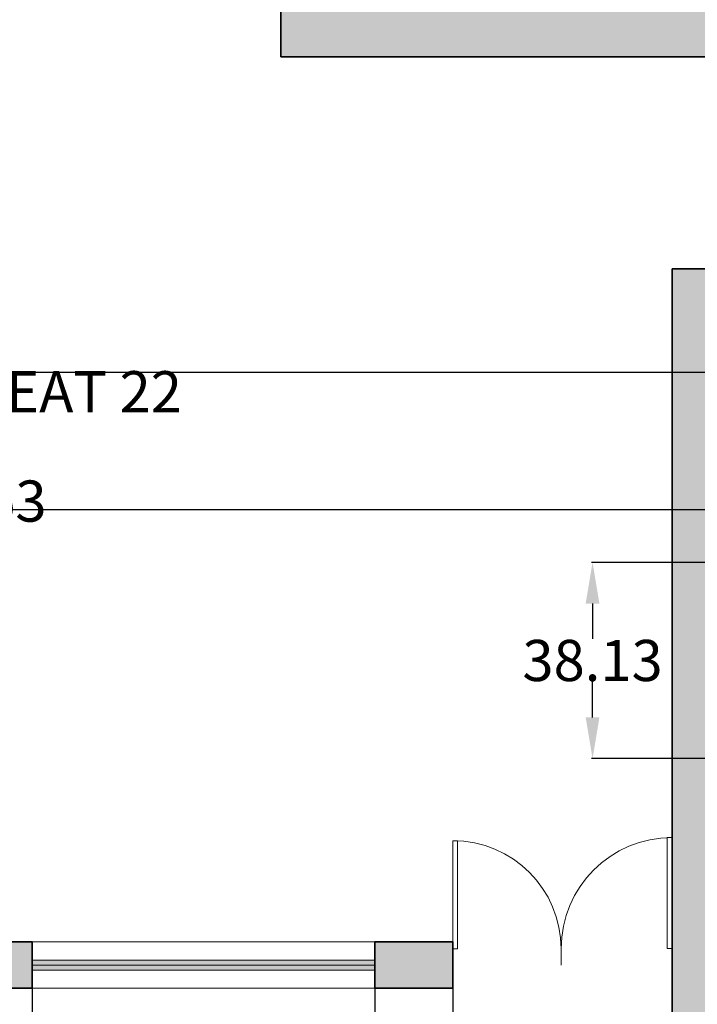
# Model space of a CAD drawing. Units: inches. Extents: x -52 to 678, y 23 to 685.
# Tile 5 of 11: x 299 to 431, y 143 to 334. Entities that reach past the tile are written whole.
import ezdxf

# ---------------------------------------------------------------- set-up
doc = ezdxf.new("R2010")
doc.units = ezdxf.units.IN
doc.header["$MEASUREMENT"] = 0
for name, color, linetype, lineweight in [('A-ANNO-DIMS', 2, 'Continuous', 18), ('A-DOOR', 3, 'Continuous', 18), ('A-GLAZ', 4, 'Continuous', 18), ('A-WALL', 7, 'Continuous', 35)]:
    doc.layers.add(name, color=color, linetype=linetype, lineweight=lineweight)
doc.layers.add('A-GLAZ-PATT', color=18, linetype='Continuous', lineweight=13, true_color=0x000000)
doc.layers.add('A-WALL-PATT', color=18, linetype='Continuous', lineweight=13, true_color=0x000000)
doc.styles.get("Standard").update_dxf_attribs({"font": 'arial.ttf'})
doc.dimstyles.get("Standard").update_dxf_attribs({"dimtxt": 8, "dimasz": 8, "dimexe": 0.18, "dimexo": 0.0625, "dimgap": 0.09, "dimtad": 0, "dimtih": 1, "dimtoh": 1, "dimdec": 0, "dimzin": 0, "dimdsep": 46, "dimlunit": 3, "dimtxsty": 'Standard', "dimcen": 0.09, "dimadec": 0, "dimazin": 0, "dimtfac": 1, "dimtdec": 0, "dimtofl": 0, "dimtmove": 0, "dimatfit": 3, "dimfxl": 1, "dimtolj": 1, "dimtzin": 0, "dimarcsym": 0})

# ---------------------------------------------------------------- blocks, each defined once
blk = doc.blocks.new('*U14')
for p, q in [((0, 0), (0, -6)), ((40, 0), (40, -6))]:
    blk.add_line(p, q)
blk.add_lwpolyline([(0, 0), (0, 40), (1.75, 40), (1.75, 0)], close=True)
blk.add_arc((0, 0), 40, 0, 90)
blk = doc.blocks.new('*D23')
at = {"layer": 'A-ANNO-DIMS', "color": 0, "lineweight": -2, "transparency": 16777216}
for p, q in [((230.34, 265.26), (230.34, 261.89)), ((252.03, 265.26), (252.03, 261.89)), ((238.34, 262.07), (244.03, 262.07)), ((252.03, 262.07), (260.03, 262.07))]:
    blk.add_line(p, q, dxfattribs=at)
at = {"layer": 'A-ANNO-DIMS', "color": 0, "transparency": 16777216}
for points in [[(238.34, 263.4), (238.34, 260.73), (230.34, 262.07)], [(244.03, 263.4), (244.03, 260.73), (252.03, 262.07)]]:
    blk.add_solid(points, dxfattribs=at)
at = {"layer": 'Defpoints', "color": 0, "transparency": 16777216}
for p in [(230.34, 265.32), (252.03, 265.32), (252.03, 262.07)]:
    blk.add_point(p, dxfattribs=at)
at = {"layer": 'A-ANNO-DIMS', "color": 0, "transparency": 16777216, "insert": (296.68, 262.07), "char_height": 8, "attachment_point": 5}
blk.add_mtext('\\A1;LOVESEAT 22', dxfattribs=at)
blk = doc.blocks.new('*D39')
at = {"layer": 'A-ANNO-DIMS', "color": 0, "lineweight": -2, "transparency": 16777216}
for p, q in [((91.61, 327.06), (91.61, 28.49)), ((575.61, 53.06), (575.61, 28.49)), ((99.61, 28.67), (324.53, 28.67)), ((567.61, 28.67), (342.68, 28.67))]:
    blk.add_line(p, q, dxfattribs=at)
at = {"layer": 'A-ANNO-DIMS', "color": 0, "transparency": 16777216}
for points in [[(99.61, 30), (99.61, 27.33), (91.61, 28.67)], [(567.61, 30), (567.61, 27.33), (575.61, 28.67)]]:
    blk.add_solid(points, dxfattribs=at)
at = {"layer": 'Defpoints', "color": 0, "transparency": 16777216}
for p in [(91.61, 327.13), (575.61, 53.13), (575.61, 28.67)]:
    blk.add_point(p, dxfattribs=at)
at = {"layer": 'A-ANNO-DIMS', "color": 0, "transparency": 16777216, "insert": (333.61, 28.67), "char_height": 8, "attachment_point": 5}
blk.add_mtext('\\A1;484', dxfattribs=at)
blk = doc.blocks.new('*D40')
at = {"layer": 'A-ANNO-DIMS', "color": 0, "lineweight": -2, "transparency": 16777216}
for p, q in [((358.67, 525.13), (600.25, 525.13)), ((600.07, 517.13), (600.07, 293.23)), ((600.07, 61.13), (600.07, 285.02)), ((575.67, 53.13), (600.25, 53.13))]:
    blk.add_line(p, q, dxfattribs=at)
at = {"layer": 'A-ANNO-DIMS', "color": 0, "transparency": 16777216}
for points in [[(598.73, 517.13), (601.4, 517.13), (600.07, 525.13)], [(598.73, 61.13), (601.4, 61.13), (600.07, 53.13)]]:
    blk.add_solid(points, dxfattribs=at)
at = {"layer": 'Defpoints', "color": 0, "transparency": 16777216}
for p in [(358.61, 525.13), (600.07, 525.13), (575.61, 53.13)]:
    blk.add_point(p, dxfattribs=at)
at = {"layer": 'A-ANNO-DIMS', "color": 0, "transparency": 16777216, "insert": (600.07, 289.13), "char_height": 8, "attachment_point": 5}
blk.add_mtext('\\A1;472', dxfattribs=at)
blk = doc.blocks.new('*D47')
at = {"layer": 'A-ANNO-DIMS', "color": 0, "lineweight": -2, "transparency": 16777216}
for p, q in [((188.54, 146.13), (66.97, 146.13)), ((67.15, 138.13), (67.15, 103.8)), ((67.15, 61.13), (67.15, 95.45)), ((425.54, 53.13), (66.97, 53.13))]:
    blk.add_line(p, q, dxfattribs=at)
at = {"layer": 'A-ANNO-DIMS', "color": 0, "transparency": 16777216}
for points in [[(65.81, 138.13), (68.48, 138.13), (67.15, 146.13)], [(65.81, 61.13), (68.48, 61.13), (67.15, 53.13)]]:
    blk.add_solid(points, dxfattribs=at)
at = {"layer": 'Defpoints', "color": 0, "transparency": 16777216}
for p in [(67.15, 146.13), (188.61, 146.13), (425.61, 53.13)]:
    blk.add_point(p, dxfattribs=at)
at = {"layer": 'A-ANNO-DIMS', "color": 0, "transparency": 16777216, "insert": (67.15, 99.63), "char_height": 8, "attachment_point": 5}
blk.add_mtext('\\A1;93', dxfattribs=at)
blk = doc.blocks.new('*D78')
at = {"layer": 'A-ANNO-DIMS', "color": 0, "lineweight": -2, "transparency": 16777216}
for p, q in [((301.27, 146.06), (301.27, 121.49)), ((367.88, 146.06), (367.88, 121.49)), ((309.27, 121.67), (321.74, 121.67)), ((359.88, 121.67), (347.41, 121.67))]:
    blk.add_line(p, q, dxfattribs=at)
at = {"layer": 'A-ANNO-DIMS', "color": 0, "transparency": 16777216}
for points in [[(309.27, 123), (309.27, 120.33), (301.27, 121.67)], [(359.88, 123), (359.88, 120.33), (367.88, 121.67)]]:
    blk.add_solid(points, dxfattribs=at)
at = {"layer": 'Defpoints', "color": 0, "transparency": 16777216}
for p in [(301.27, 146.13), (367.88, 146.13), (301.27, 121.67)]:
    blk.add_point(p, dxfattribs=at)
at = {"layer": 'A-ANNO-DIMS', "color": 0, "transparency": 16777216, "insert": (334.58, 121.67), "char_height": 8, "attachment_point": 5}
blk.add_mtext('\\A1;66.61', dxfattribs=at)
blk = doc.blocks.new('*D79')
at = {"layer": 'A-ANNO-DIMS', "color": 0, "lineweight": -2, "transparency": 16777216}
for p, q in [((383, 153.72), (383.04, 129.14)), ((425.61, 153.8), (425.65, 129.22)), ((391.04, 129.34), (391.37, 129.34)), ((417.65, 129.39), (417.32, 129.38))]:
    blk.add_line(p, q, dxfattribs=at)
at = {"layer": 'A-ANNO-DIMS', "color": 0, "transparency": 16777216}
for points in [[(391.04, 130.67), (391.05, 128), (383.04, 129.32)], [(417.65, 130.72), (417.65, 128.05), (425.65, 129.4)]]:
    blk.add_solid(points, dxfattribs=at)
at = {"layer": 'Defpoints', "color": 0, "transparency": 16777216}
for p in [(383, 153.78), (425.61, 153.86), (383.04, 129.32)]:
    blk.add_point(p, dxfattribs=at)
at = {"layer": 'A-ANNO-DIMS', "color": 0, "transparency": 16777216, "insert": (404.35, 129.36), "char_height": 8, "attachment_point": 5}
blk.add_mtext('\\A1;42.61', dxfattribs=at)
blk = doc.blocks.new('*D80')
at = {"layer": 'A-ANNO-DIMS', "color": 0, "lineweight": -2, "transparency": 16777216}
for p, q in [((367.88, 146.06), (367.88, 121.49)), ((383, 146.06), (383, 121.49)), ((359.88, 121.67), (351.88, 121.67)), ((391, 121.67), (399, 121.67))]:
    blk.add_line(p, q, dxfattribs=at)
at = {"layer": 'A-ANNO-DIMS', "color": 0, "transparency": 16777216}
for points in [[(359.88, 123), (359.88, 120.33), (367.88, 121.67)], [(391, 123), (391, 120.33), (383, 121.67)]]:
    blk.add_solid(points, dxfattribs=at)
at = {"layer": 'Defpoints', "color": 0, "transparency": 16777216}
for p in [(367.88, 146.13), (383, 146.13), (367.88, 121.67)]:
    blk.add_point(p, dxfattribs=at)
at = {"layer": 'A-ANNO-DIMS', "color": 0, "transparency": 16777216, "insert": (335.56, 121.67), "char_height": 8, "attachment_point": 5}
blk.add_mtext('\\A1;15.117', dxfattribs=at)
blk = doc.blocks.new('*D98')
at = {"layer": 'A-ANNO-DIMS', "color": 0, "lineweight": -2, "transparency": 16777216}
for p, q in [((434.54, 228.91), (409.97, 228.91)), ((410.15, 220.91), (410.15, 214.02)), ((410.15, 198.77), (410.15, 205.66)), ((434.54, 190.77), (409.97, 190.77))]:
    blk.add_line(p, q, dxfattribs=at)
at = {"layer": 'A-ANNO-DIMS', "color": 0, "transparency": 16777216}
for points in [[(408.81, 220.91), (411.48, 220.91), (410.15, 228.91)], [(408.81, 198.77), (411.48, 198.77), (410.15, 190.77)]]:
    blk.add_solid(points, dxfattribs=at)
at = {"layer": 'Defpoints', "color": 0, "transparency": 16777216}
for p in [(410.15, 228.91), (434.61, 228.91), (434.61, 190.77)]:
    blk.add_point(p, dxfattribs=at)
at = {"layer": 'A-ANNO-DIMS', "color": 0, "transparency": 16777216, "insert": (410.15, 209.84), "char_height": 8, "attachment_point": 5}
blk.add_mtext('\\A1;38.13', dxfattribs=at)
blk = doc.blocks.new('*D100')
at = {"layer": 'A-ANNO-DIMS', "color": 0, "lineweight": -2, "transparency": 16777216}
for p, q in [((519.99, 265.81), (66.97, 265.81)), ((67.15, 257.81), (67.15, 256.65)), ((67.15, 247.13), (67.15, 248.3)), ((521.98, 239.13), (66.97, 239.13))]:
    blk.add_line(p, q, dxfattribs=at)
at = {"layer": 'A-ANNO-DIMS', "color": 0, "transparency": 16777216}
for points in [[(65.81, 257.81), (68.48, 257.81), (67.15, 265.81)], [(65.81, 247.13), (68.48, 247.13), (67.15, 239.13)]]:
    blk.add_solid(points, dxfattribs=at)
at = {"layer": 'Defpoints', "color": 0, "transparency": 16777216}
for p in [(520.05, 265.81), (67.15, 239.13), (522.04, 239.13)]:
    blk.add_point(p, dxfattribs=at)
at = {"layer": 'A-ANNO-DIMS', "color": 0, "transparency": 16777216, "insert": (67.15, 252.47), "char_height": 8, "attachment_point": 5}
blk.add_mtext('\\A1;26.69', dxfattribs=at)
blk = doc.blocks.new('*D102')
at = {"layer": 'A-ANNO-DIMS', "color": 0, "lineweight": -2, "transparency": 16777216}
for p, q in [((266.04, 271.64), (290.62, 271.64)), ((290.44, 263.64), (290.44, 245)), ((290.44, 218.01), (290.44, 236.65)), ((266.04, 210.01), (290.62, 210.01))]:
    blk.add_line(p, q, dxfattribs=at)
at = {"layer": 'A-ANNO-DIMS', "color": 0, "transparency": 16777216}
for points in [[(289.1, 263.64), (291.77, 263.64), (290.44, 271.64)], [(289.1, 218.01), (291.77, 218.01), (290.44, 210.01)]]:
    blk.add_solid(points, dxfattribs=at)
at = {"layer": 'Defpoints', "color": 0, "transparency": 16777216}
for p in [(265.98, 271.64), (265.98, 210.01), (290.44, 210.01)]:
    blk.add_point(p, dxfattribs=at)
at = {"layer": 'A-ANNO-DIMS', "color": 0, "transparency": 16777216, "insert": (290.44, 240.82), "char_height": 8, "attachment_point": 5}
blk.add_mtext('\\A1;61.63', dxfattribs=at)
blk = doc.blocks.new('*D104')
at = {"layer": 'A-ANNO-DIMS', "color": 0, "lineweight": -2, "transparency": 16777216}
for p, q in [((265.91, 210.01), (66.97, 210.01)), ((67.15, 202.01), (67.15, 186.74)), ((67.15, 163.13), (67.15, 178.39)), ((301.21, 155.13), (66.97, 155.13))]:
    blk.add_line(p, q, dxfattribs=at)
at = {"layer": 'A-ANNO-DIMS', "color": 0, "transparency": 16777216}
for points in [[(65.81, 202.01), (68.48, 202.01), (67.15, 210.01)], [(65.81, 163.13), (68.48, 163.13), (67.15, 155.13)]]:
    blk.add_solid(points, dxfattribs=at)
at = {"layer": 'Defpoints', "color": 0, "transparency": 16777216}
for p in [(265.98, 210.01), (67.15, 155.13), (301.27, 155.13)]:
    blk.add_point(p, dxfattribs=at)
at = {"layer": 'A-ANNO-DIMS', "color": 0, "transparency": 16777216, "insert": (67.15, 182.57), "char_height": 8, "attachment_point": 5}
blk.add_mtext('\\A1;54.89', dxfattribs=at)

msp = doc.modelspace()

# ---------------------------------------------------------------- hatches: boundary and pattern name
at = {"layer": 'A-GLAZ-PATT'}
h = msp.add_hatch(color=256, dxfattribs=at)
h.dxf.hatch_style = 1
h.paths.add_polyline_path([(301.2728, 151.6267), (301.2728, 150.6267), (367.8819, 150.6267), (367.8819, 151.6267)])
h = msp.add_hatch(color=256, dxfattribs=at)
h.dxf.hatch_style = 1
h.paths.add_polyline_path([(367.8819, 149.6267), (367.8819, 150.6267), (301.2728, 150.6267), (301.2728, 149.6267)])
at = {"layer": 'A-WALL-PATT'}
h = msp.add_hatch(color=256, dxfattribs=at)
h.dxf.hatch_style = 1
h.paths.add_polyline_path([(349.6053, 340.107), (349.6053, 327.1267), (410.6053, 327.1267), (434.6053, 327.1267), (434.6053, 336.1267), (410.6053, 336.1267), (410.6053, 340.107), (410.6053, 363.4905), (406.6053, 363.4905), (406.6053, 340.107), (406.6053, 336.1267), (358.6053, 336.1267), (358.6053, 340.107), (358.6053, 392.1267), (382.6053, 392.1267), (382.6053, 396.1267), (358.6053, 396.1267), (358.6053, 468.1267), (372.5751, 468.1267), (372.5751, 477.1267), (358.6053, 477.1267), (358.6053, 525.1267), (341.0247, 525.1267), (341.0247, 516.1267), (349.6053, 516.1267)])
h = msp.add_hatch(color=256, dxfattribs=at)
h.dxf.hatch_style = 1
h.paths.add_polyline_path([(434.6053, 239.1267), (434.6053, 285.9421), (425.6053, 285.9421), (425.6053, 239.1267), (425.6053, 53.1267), (468.8253, 53.1267), (468.8253, 62.1267), (434.6053, 62.1267)])
h = msp.add_hatch(color=256, dxfattribs=at)
h.dxf.hatch_style = 1
h.paths.add_polyline_path([(301.2728, 146.1267), (301.2728, 155.1267), (197.6053, 155.1267), (197.6053, 159.3213), (188.6053, 159.3213), (188.6053, 146.1267)])
h = msp.add_hatch(color=256, dxfattribs=at)
h.dxf.hatch_style = 1
h.paths.add_polyline_path([(367.8819, 155.1267), (367.8819, 146.1267), (382.9989, 146.1267), (382.9989, 155.1267)])

# ---------------------------------------------------------------- linework, layer by layer
at = {"layer": 'A-GLAZ'}
for p, q in [((301.2728, 155.1267), (367.8819, 155.1267)), ((301.2728, 151.6267), (367.8819, 151.6267)), ((301.2728, 150.6267), (367.8819, 150.6267)), ((301.2728, 149.6267), (367.8819, 149.6267)), ((301.2728, 146.1267), (367.8819, 146.1267))]:
    msp.add_line(p, q, dxfattribs=at)
at = {"layer": 'A-WALL'}
for p, q in [((349.6053, 340.107), (349.6053, 327.1267)), ((410.6053, 327.1267), (349.6053, 327.1267)), ((410.6053, 327.1267), (434.6053, 327.1267)), ((434.6053, 285.9421), (425.6053, 285.9421)), ((425.6053, 285.9421), (425.6053, 239.1267)), ((425.6053, 53.1267), (425.6053, 239.1267)), ((197.6053, 155.1267), (301.2728, 155.1267)), ((301.2728, 155.1267), (301.2728, 146.1267)), ((367.8819, 146.1267), (367.8819, 155.1267)), ((367.8819, 155.1267), (382.9989, 155.1267)), ((382.9989, 155.1267), (382.9989, 146.1267)), ((188.6053, 146.1267), (301.2728, 146.1267)), ((367.8819, 146.1267), (382.9989, 146.1267))]:
    msp.add_line(p, q, dxfattribs=at)

# ---------------------------------------------------------------- block references
at = {"layer": 'A-DOOR'}
for p, xscale, yscale, zscale in [((382.9989, 153.7824), 0.5259416425726818, 0.5259416425726818, 0.5259416425726818), ((425.6053, 153.86), -0.5388829540515353, 0.5388829540515353, 0.5388829540515353)]:
    msp.add_blockref('*U14', p, dxfattribs=dict(at, xscale=xscale, yscale=yscale, zscale=zscale))

# ---------------------------------------------------------------- dimensions: what is measured, and where the dimension line sits
at = {"layer": 'A-ANNO-DIMS'}
for base, p1, p2, angle, override, picture, middle in [((600.0653, 525.1267), (575.6053, 53.1267), (358.6053, 525.1267), 90, {"dimdec": 0, "dimlfac": 1, "dimrnd": 0, "dimzin": 0, "dimdsep": 46, "dimlunit": 2}, '*D40', (600.0653, 289.1267)), ((290.4363, 210.0118), (265.9763, 271.638), (265.9763, 210.0118), 270, {"dimdec": 2, "dimlfac": 1, "dimrnd": 0, "dimzin": 0, "dimdsep": 46, "dimlunit": 2}, '*D102', (290.4363, 240.8249)), ((67.1453, 239.1267), (520.0511, 265.8145), (522.0448, 239.1267), 90, {"dimdec": 2, "dimlfac": 1, "dimrnd": 0, "dimzin": 0, "dimdsep": 46, "dimlunit": 2}, '*D100', (67.1453, 252.4706)), ((410.1453, 228.9068), (434.6053, 190.774), (434.6053, 228.9068), 90, {"dimdec": 2, "dimlfac": 1, "dimrnd": 0, "dimzin": 0, "dimdsep": 46, "dimlunit": 2}, '*D98', (410.1453, 209.8404)), ((67.1453, 155.1267), (265.9763, 210.0118), (301.2728, 155.1267), 90, {"dimdec": 2, "dimlfac": 1, "dimrnd": 0, "dimzin": 0, "dimdsep": 46, "dimlunit": 2}, '*D104', (67.1453, 182.5693)), ((383.0434, 129.3224), (425.6053, 153.86), (382.9989, 153.7824), 180.104418, {"dimdec": 2, "dimlfac": 1, "dimrnd": 0, "dimzin": 0, "dimdsep": 46, "dimlunit": 2}, '*D79', (404.3466, 129.3613)), ((67.1453, 146.1267), (425.6053, 53.1267), (188.6053, 146.1267), 90, {"dimdec": 0, "dimlfac": 1, "dimrnd": 0, "dimzin": 0, "dimdsep": 46, "dimlunit": 2}, '*D47', (67.1453, 99.6267)), ((301.2728, 121.6667), (367.8819, 146.1267), (301.2728, 146.1267), 180, {"dimdec": 2, "dimlfac": 1, "dimrnd": 0, "dimzin": 0, "dimdsep": 46, "dimlunit": 2}, '*D78', (334.5773, 121.6667)), ((367.8819, 121.6667), (382.9989, 146.1267), (367.8819, 146.1267), 180, {"dimdec": 3, "dimlfac": 1, "dimrnd": 0, "dimzin": 0, "dimdsep": 46, "dimlunit": 2}, '*D80', (335.5627, 121.6667))]:
    dim = msp.add_linear_dim(base=base, p1=p1, p2=p2, angle=angle, dimstyle='Standard', override=override, dxfattribs=at)
    dim.commit()
    dim.dimension.update_dxf_attribs({"geometry": picture, "text_midpoint": middle})
dim = msp.add_linear_dim(base=(575.6053, 28.6667), p1=(91.6053, 327.1267), p2=(575.6053, 53.1267), dimstyle='Standard', override={"dimdec": 0, "dimlfac": 1, "dimrnd": 0, "dimzin": 0, "dimdsep": 46, "dimlunit": 2}, dxfattribs=at)
dim.commit()
dim.dimension.update_dxf_attribs({"geometry": '*D39', "text_midpoint": (333.6053, 28.6667)})
dim = msp.add_linear_dim(base=(252.0267, 262.0679), p1=(230.3425, 265.3206), p2=(252.0267, 265.3206), text='LOVESEAT <>', dimstyle='Standard', override={"dimdec": 0, "dimlfac": 1, "dimrnd": 0, "dimzin": 0, "dimdsep": 46, "dimlunit": 2}, dxfattribs=at)
dim.commit()
dim.dimension.update_dxf_attribs({"geometry": '*D23', "text_midpoint": (296.6842, 262.0679)})

doc.saveas('drawing.dxf')
